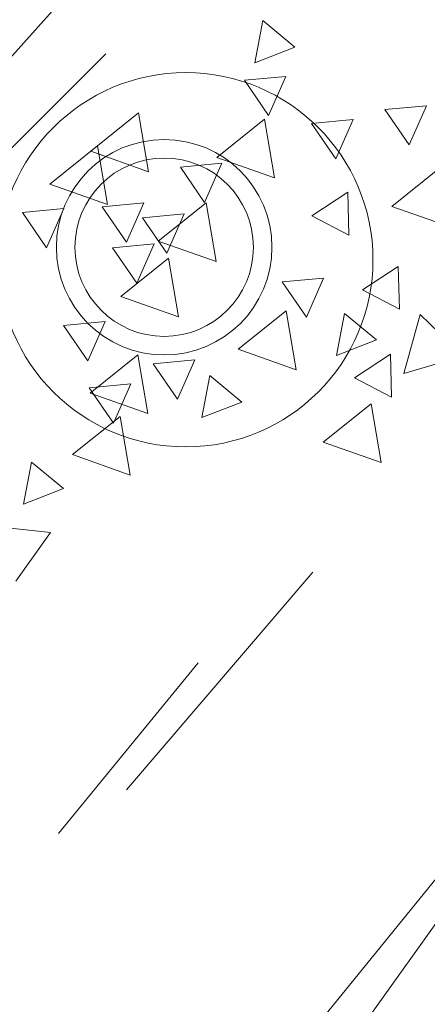
# Model space of a CAD drawing. Units: inches. Extents: x 375 to 1122, y 27 to 1069.
# Tile 27 of 155: x 721 to 732, y 271 to 297. Entities that reach past the tile are written whole.
import ezdxf

# ---------------------------------------------------------------- set-up
doc = ezdxf.new("R2010")
doc.units = ezdxf.units.IN
doc.layers.add('Furniture', color=30, linetype='Continuous', lineweight=18)

# ---------------------------------------------------------------- blocks, each defined once
blk = doc.blocks.new('A$C403C54AD')
for p, q in [((1.43807, 1.16281, -0.0006), (1.46553, 1.19082, -0.0006)), ((1.46553, 1.19082, -0.0006), (1.47699, 1.15208, -0.0006)), ((1.78922, 1.18993, 0.03663), (1.95298, 1.05694, 0.03663)), ((1.38035, 1.18225, -0.0006), (1.36693, 1.14415, -0.0006)), ((1.36693, 1.14415, -0.0006), (1.34169, 1.17565, -0.0006)), ((1.83016, 1.1797, 0.03663), (1.90181, 1.12855, 0.03663)), ((0.95931, 1.17062, -0.0006), (1.35847, 0.81256, -0.0006)), ((1.30057, 1.1669, -0.0006), (1.32646, 1.15553, -0.0006)), ((1.30314, 1.13957, -0.0006), (1.30057, 1.1669, -0.0006)), ((1.47699, 1.15208, -0.0006), (1.43807, 1.16281, -0.0006)), ((1.32646, 1.15553, -0.0006), (1.30314, 1.13957, -0.0006)), ((1.40642, 1.1484, -0.0006), (1.43467, 1.14912, -0.0006)), ((1.43467, 1.14912, -0.0006), (1.42197, 1.12477, -0.0006)), ((1.42197, 1.12477, -0.0006), (1.40642, 1.1484, -0.0006)), ((1.46436, 1.14322, -0.0006), (1.49261, 1.14394, -0.0006)), ((1.47991, 1.1196, -0.0006), (1.46436, 1.14322, -0.0006)), ((1.49261, 1.14394, -0.0006), (1.47991, 1.1196, -0.0006)), ((1.49708, 1.13054, -0.0006), (1.53574, 1.13714, -0.0006)), ((1.53574, 1.13714, -0.0006), (1.52232, 1.09903, -0.0006)), ((1.43741, 1.11297, -0.0006), (1.45492, 1.13412, -0.0006)), ((1.45492, 1.13412, -0.0006), (1.46519, 1.10777, -0.0006)), ((1.52232, 1.09903, -0.0006), (1.49708, 1.13054, -0.0006)), ((1.31226, 1.09126, -0.0006), (1.30969, 1.1186, -0.0006)), ((1.30969, 1.1186, -0.0006), (1.33558, 1.10722, -0.0006)), ((1.35757, 1.11509, -0.0006), (1.38582, 1.11581, -0.0006)), ((1.37311, 1.09147, -0.0006), (1.35757, 1.11509, -0.0006)), ((1.38582, 1.11581, -0.0006), (1.37311, 1.09147, -0.0006)), ((1.46519, 1.10777, -0.0006), (1.43741, 1.11297, -0.0006)), ((1.33558, 1.10722, -0.0006), (1.31226, 1.09126, -0.0006)), ((1.41669, 1.07191, -0.0006), (1.41412, 1.09924, -0.0006)), ((1.41412, 1.09924, -0.0006), (1.44001, 1.08787, -0.0006)), ((1.608, 1.0922, -0.0006), (1.75129, 0.96944, -0.0006)), ((1.44001, 1.08787, -0.0006), (1.41669, 1.07191, -0.0006)), ((1.24444, 1.05916, -0.0006), (1.26195, 1.08031, -0.0006)), ((1.26195, 1.08031, -0.0006), (1.27222, 1.05396, -0.0006)), ((1.43585, 1.07454, -0.0006), (1.47452, 1.08115, -0.0006)), ((1.47452, 1.08115, -0.0006), (1.4611, 1.04304, -0.0006)), ((1.28381, 1.04703, -0.0006), (1.28124, 1.07437, -0.0006)), ((1.28124, 1.07437, -0.0006), (1.30713, 1.06299, -0.0006)), ((1.4611, 1.04304, -0.0006), (1.43585, 1.07454, -0.0006)), ((1.30948, 1.06033, -0.0006), (1.34815, 1.06694, -0.0006)), ((1.34815, 1.06694, -0.0006), (1.33473, 1.02883, -0.0006)), ((1.27222, 1.05396, -0.0006), (1.24444, 1.05916, -0.0006)), ((1.30713, 1.06299, -0.0006), (1.28381, 1.04703, -0.0006)), ((1.33473, 1.02883, -0.0006), (1.30948, 1.06033, -0.0006)), ((1.47832, 1.02428, -0.0006), (1.49583, 1.04543, -0.0006)), ((1.49583, 1.04543, -0.0006), (1.5061, 1.01907, -0.0006)), ((1.34102, 1.00487, -0.0006), (1.33845, 1.03221, -0.0006)), ((1.33845, 1.03221, -0.0006), (1.36435, 1.02083, -0.0006)), ((1.36461, 1.02181, -0.0006), (1.40328, 1.02841, -0.0006)), ((1.40328, 1.02841, -0.0006), (1.38985, 0.99031, -0.0006)), ((1.36435, 1.02083, -0.0006), (1.34102, 1.00487, -0.0006)), ((1.38985, 0.99031, -0.0006), (1.36461, 1.02181, -0.0006)), ((1.5061, 1.01907, -0.0006), (1.47832, 1.02428, -0.0006)), ((1.47068, 0.98703, -0.0006), (1.46811, 1.01437, -0.0006)), ((1.46811, 1.01437, -0.0006), (1.494, 1.00299, -0.0006)), ((1.66765, 1.0166, -0.0006), (1.78023, 0.92452, -0.0006)), ((1.3745, 0.97999, -0.0006), (1.37193, 1.00733, -0.0006)), ((1.37193, 1.00733, -0.0006), (1.39782, 0.99596, -0.0006)), ((1.40106, 0.9971, -0.0006), (1.43972, 1.00371, -0.0006)), ((1.43972, 1.00371, -0.0006), (1.4263, 0.9656, -0.0006)), ((1.494, 1.00299, -0.0006), (1.47068, 0.98703, -0.0006)), ((1.39782, 0.99596, -0.0006), (1.3745, 0.97999, -0.0006)), ((1.4263, 0.9656, -0.0006), (1.40106, 0.9971, -0.0006)), ((1.39427, 0.96028, -0.0006), (1.3917, 0.98762, -0.0006)), ((1.3917, 0.98762, -0.0006), (1.41759, 0.97624, -0.0006)), ((1.30537, 0.97738, -0.0006), (1.34404, 0.98398, -0.0006)), ((1.34404, 0.98398, -0.0006), (1.33062, 0.94587, -0.0006)), ((1.36711, 0.95348, -0.0006), (1.36453, 0.98082, -0.0006)), ((1.36453, 0.98082, -0.0006), (1.39043, 0.96944, -0.0006)), ((1.46471, 0.97689, -0.0006), (1.50337, 0.9835, -0.0006)), ((1.50337, 0.9835, -0.0006), (1.48995, 0.94539, -0.0006)), ((1.33062, 0.94587, -0.0006), (1.30537, 0.97738, -0.0006)), ((1.41759, 0.97624, -0.0006), (1.39427, 0.96028, -0.0006)), ((1.48995, 0.94539, -0.0006), (1.46471, 0.97689, -0.0006)), ((1.39043, 0.96944, -0.0006), (1.36711, 0.95348, -0.0006)), ((1.48643, 0.9449, -0.0006), (1.48386, 0.97224, -0.0006)), ((1.48386, 0.97224, -0.0006), (1.50975, 0.96086, -0.0006)), ((1.50527, 0.96524, -0.0006), (1.54394, 0.97185, -0.0006)), ((1.54394, 0.97185, -0.0006), (1.53052, 0.93374, -0.0006)), ((1.50975, 0.96086, -0.0006), (1.48643, 0.9449, -0.0006)), ((1.53052, 0.93374, -0.0006), (1.50527, 0.96524, -0.0006)), ((1.26636, 0.95578, -0.0006), (1.37894, 0.84325, -0.0006)), ((1.32706, 0.95032, -0.0006), (1.36572, 0.95693, -0.0006)), ((1.36572, 0.95693, -0.0006), (1.3523, 0.91882, -0.0006)), ((1.44544, 0.92794, -0.0006), (1.44286, 0.95528, -0.0006)), ((1.44286, 0.95528, -0.0006), (1.46876, 0.9439, -0.0006)), ((1.3523, 0.91882, -0.0006), (1.32706, 0.95032, -0.0006)), ((1.46876, 0.9439, -0.0006), (1.44544, 0.92794, -0.0006)), ((1.37092, 0.9008, -0.0006), (1.36834, 0.92814, -0.0006)), ((1.36834, 0.92814, -0.0006), (1.39424, 0.91676, -0.0006)), ((1.5354, 0.90675, -0.0006), (1.55291, 0.9279, -0.0006)), ((1.55291, 0.9279, -0.0006), (1.56317, 0.90154, -0.0006)), ((1.39424, 0.91676, -0.0006), (1.37092, 0.9008, -0.0006)), ((1.57741, 0.87913, -0.0006), (1.58183, 0.91926, -0.0006)), ((1.58183, 0.91926, -0.0006), (1.61385, 0.89659, -0.0006)), ((1.56317, 0.90154, -0.0006), (1.5354, 0.90675, -0.0006))]:
    blk.add_line(p, q)
for centre, radius in [((1.40208, 1.00844, -0.0006), 0.12331), ((1.39383, 0.99423, -0.0006), 0.07097), ((1.39383, 0.99423, -0.0006), 0.05876)]:
    blk.add_circle(centre, radius)

msp = doc.modelspace()

# ---------------------------------------------------------------- block references
at = {"layer": 'Furniture', "xscale": 39.9918517141215, "yscale": 39.9918517141215, "zscale": 39.9918517141215, "rotation": 270}
msp.add_blockref('A$C403C54AD', (684.955, 346.287, 0.024), dxfattribs=at)

doc.saveas('drawing.dxf')
